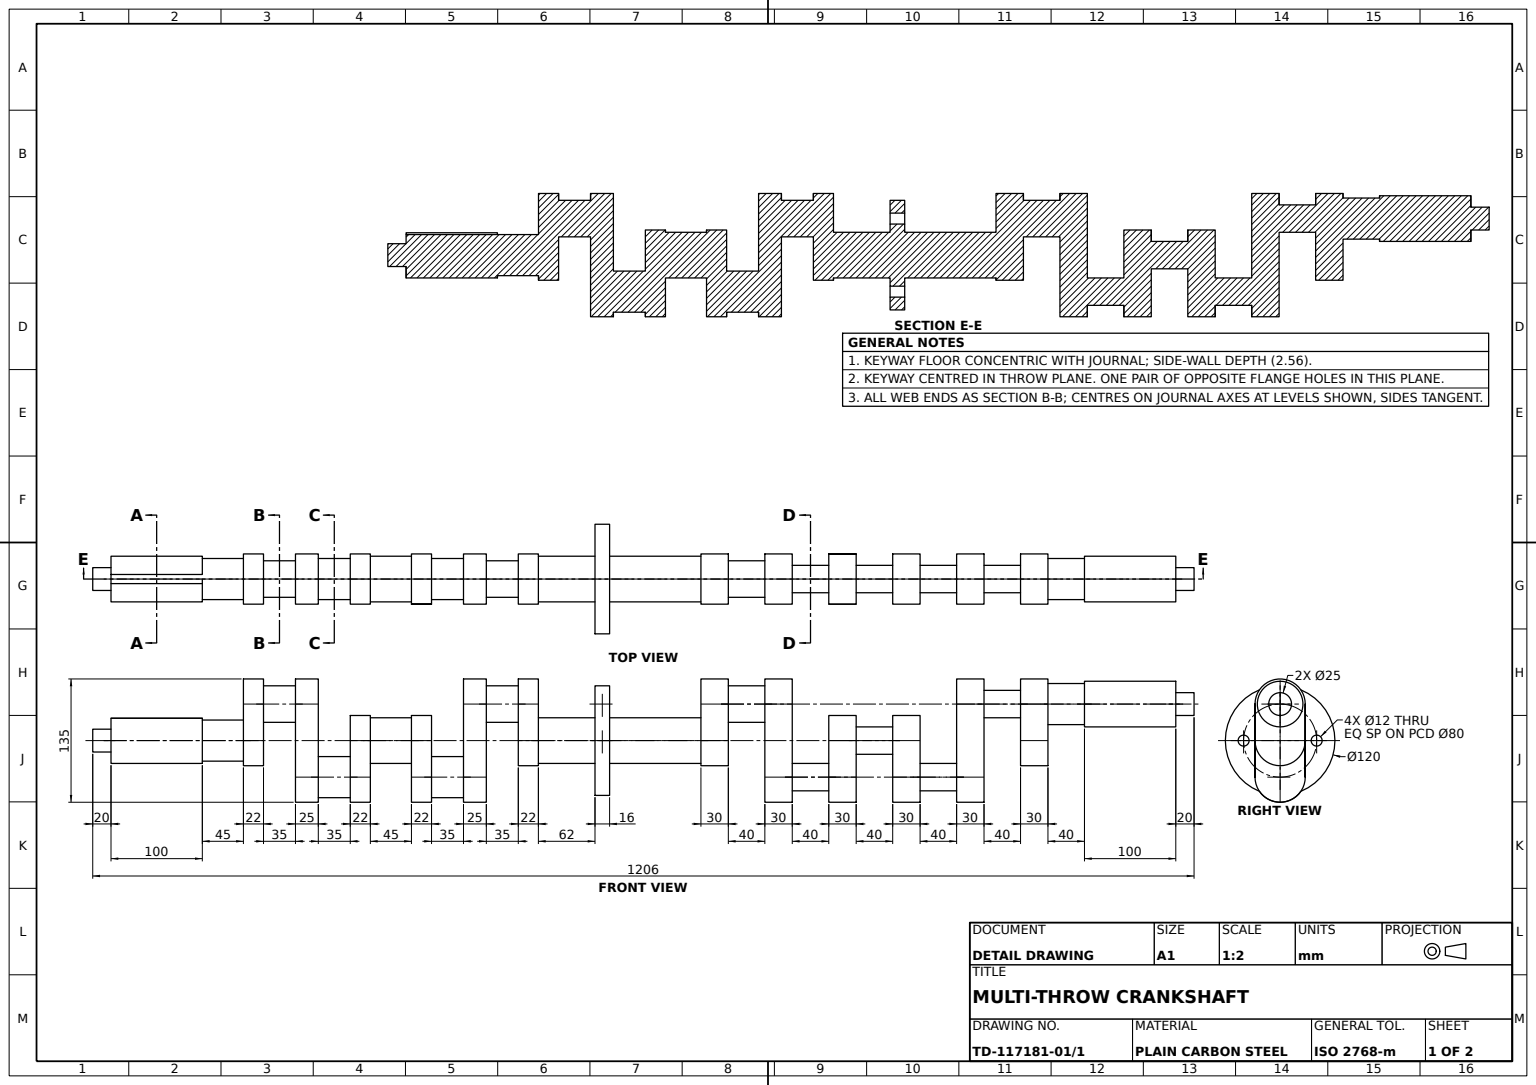
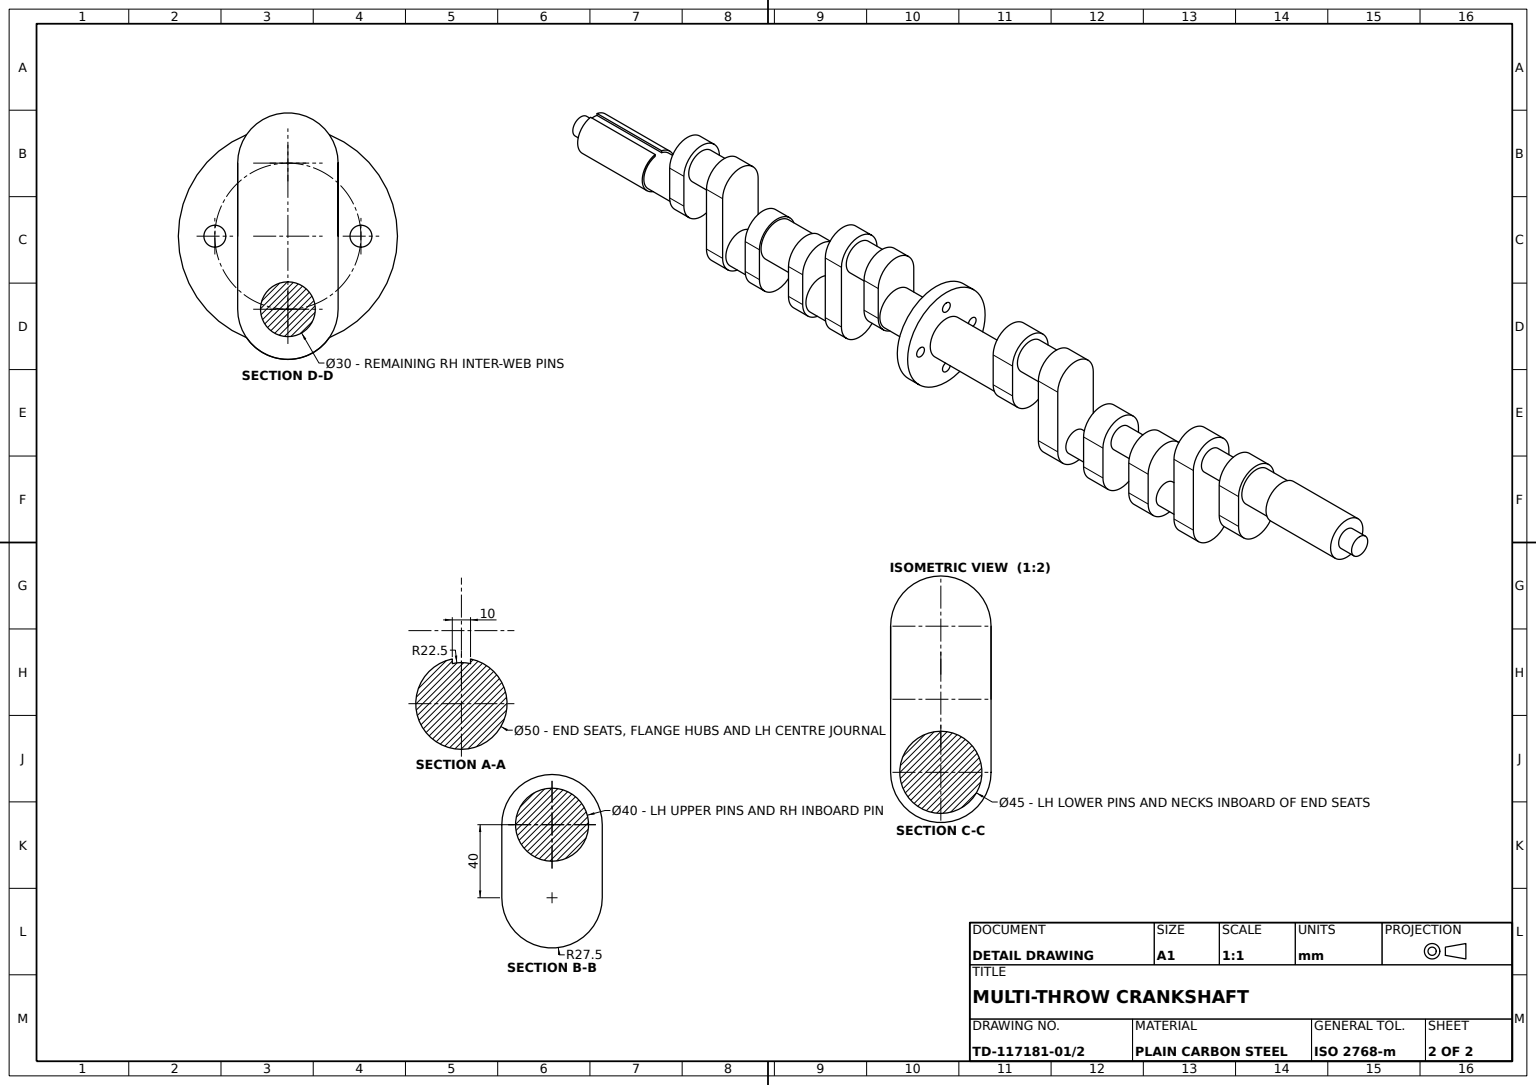
SolidWorks part; units mm, degrees
other "Markup1"
sketch "Sketch6"
material "Plain Carbon Steel"
ref_plane "Front Plane" through (0, 0, 0) normal (0, 0, 1) x (1, 0, 0)
ref_plane "Top Plane" through (0, 0, 0) normal (0, 1, 0) x (1, 0, 0)
ref_plane "Right Plane" through (0, 0, 0) normal (1, 0, 0) x (0, 0, -1)
sketch "Centre Flange Sketch" plane through (0, 0, 0) normal (0, 0, 1) x (1, 0, 0)
  circle A0 centre (0, 0) radius 60
  dimension "D1" = 120
extrude "Centre Flange Ø120" add sketch "Centre Flange Sketch" along normal blind 16
sketch "Flange Holes Sketch" plane through (0, 0, 16) normal (0, 0, 1) x (1, 0, 0)
  line L0 (0, 60) -> (0, -60) construction
  line L1 (-60, 0) -> (60, 0) construction
  circle A1 centre (0, 0) radius 60 construction
  circle A2 centre (0, 40) radius 6
  circle A3 centre (40, 0) radius 6
  circle A4 centre (0, -40) radius 6
  circle A5 centre (-40, 0) radius 6
  point P1 (0, 0)
  dimension "D1" = 40
  dimension "D2" = 12
  dimension "D3" = 40
  dimension "D4" = 40
  dimension "D5" = 40
extrude "Flange Holes Ø12" cut sketch "Flange Holes Sketch" against normal through all
sketch "A Journal 1 Sketch" plane through (0, 0, 16) normal (0, 0, 1) x (1, 0, 0)
  circle A0 centre (0, 0) radius 25
  dimension "D1" = 50
extrude "A Journal 1 Ø50" add sketch "A Journal 1 Sketch" along normal blind 62
sketch "A Web 1 Sketch" plane through (0, 0, 78) normal (0, 0, 1) x (1, 0, 0)
  line L0 (0, 0) -> (-40, 0) construction
  line L1 (0, -27.5) -> (-40, -27.5)
  line L2 (0, 27.5) -> (-40, 27.5)
  arc A0 (0, -27.5) -> (0, 27.5) centre (0, 0) ccw
  arc A1 (-40, 27.5) -> (-40, -27.5) centre (-40, 0) ccw
  point P3 (-20, 0)
  dimension "D2" = 27.5
  dimension "D1" = 40
extrude "A Web 1" add sketch "A Web 1 Sketch" along normal blind 22
sketch "A Pin 1 Sketch" plane through (0, 0, 100) normal (0, 0, 1) x (1, 0, 0)
  line L0 (-40, -27.5) -> (-40, 27.5) construction
  circle A0 centre (-40, 0) radius 20
  dimension "D1" = 40
extrude "A Pin 1 Ø40" add sketch "A Pin 1 Sketch" along normal blind 35
sketch "A Web 2 Sketch" plane through (0, 0, 135) normal (0, 0, 1) x (1, 0, 0)
  line L0 (-40, 0) -> (40, 0) construction
  line L1 (-40, 27.5) -> (40, 27.5)
  line L2 (-40, -27.5) -> (40, -27.5)
  arc A0 (-40, 27.5) -> (-40, -27.5) centre (-40, 0) ccw
  arc A1 (40, -27.5) -> (40, 27.5) centre (40, 0) ccw
  point P4 (0, 0)
  dimension "D2" = 27.5
  dimension "D1" = 80
extrude "A Web 2" add sketch "A Web 2 Sketch" along normal blind 25
sketch "A Pin 2 Sketch" plane through (0, 0, 160) normal (0, 0, 1) x (1, 0, 0)
  line L0 (40, 27.5) -> (40, -27.5) construction
  arc A0 (40, -27.5) -> (40, 27.5) centre (40, 0) ccw construction
  circle A1 centre (40, 0) radius 22.5
  dimension "D1" = 45
  dimension "D2" = 40
extrude "A Pin 2 Ø45" add sketch "A Pin 2 Sketch" along normal blind 35
sketch "A Web 3 Sketch" plane through (0, 0, 195) normal (0, 0, 1) x (1, 0, 0)
  line L0 (40, 0) -> (0, 0) construction
  line L1 (40, -27.5) -> (0, -27.5)
  line L2 (40, 27.5) -> (0, 27.5)
  arc A0 (40, -27.5) -> (40, 27.5) centre (40, 0) ccw
  arc A1 (0, 27.5) -> (0, -27.5) centre (0, 0) ccw
  point P4 (20, 0)
  dimension "D2" = 27.5
  dimension "D1" = 40
extrude "A Web 3" add sketch "A Web 3 Sketch" along normal blind 22
sketch "A Journal 2 Sketch" plane through (0, 0, 217) normal (0, 0, 1) x (1, 0, 0)
  circle A0 centre (0, 0) radius 25
  dimension "D1" = 50
extrude "A Journal 2 Ø50" add sketch "A Journal 2 Sketch" along normal blind 45
sketch "A Web 4 Sketch" plane through (0, 0, 262) normal (0, 0, 1) x (1, 0, 0)
  line L0 (0, 0) -> (40, 0) construction
  line L1 (0, 27.5) -> (40, 27.5)
  line L2 (0, -27.5) -> (40, -27.5)
  arc A0 (0, 27.5) -> (0, -27.5) centre (0, 0) ccw
  arc A1 (40, -27.5) -> (40, 27.5) centre (40, 0) ccw
  point P3 (20, 0)
  dimension "D2" = 27.5
  dimension "D1" = 40
extrude "A Web 4" add sketch "A Web 4 Sketch" along normal blind 22
sketch "A Pin 3 Sketch" plane through (0, 0, 284) normal (0, 0, 1) x (1, 0, 0)
  line L0 (40, 27.5) -> (40, -27.5) construction
  line L1 (0, -27.5) -> (40, -27.5) construction
  arc A0 (40, -27.5) -> (40, 27.5) centre (40, 0) ccw construction
  circle A1 centre (40, 0) radius 22.5
  dimension "D1" = 45
extrude "A Pin 3 Ø45" add sketch "A Pin 3 Sketch" along normal blind 35
sketch "A Web 5 Sketch" plane through (0, 0, 319) normal (0, 0, 1) x (1, 0, 0)
  line L0 (40, 0) -> (-40, 0) construction
  line L1 (40, -27.5) -> (-40, -27.5)
  line L2 (40, 27.5) -> (-40, 27.5)
  arc A0 (40, -27.5) -> (40, 27.5) centre (40, 0) ccw
  arc A1 (-40, 27.5) -> (-40, -27.5) centre (-40, 0) ccw
  point P3 (0, 0)
  dimension "D2" = 27.5
  dimension "D1" = 80
extrude "A Web 5" add sketch "A Web 5 Sketch" along normal blind 25
sketch "A Pin 4 Sketch" plane through (0, 0, 344) normal (0, 0, 1) x (1, 0, 0)
  line L0 (-40, 27.5) -> (-40, -27.5) construction
  arc A0 (-40, 27.5) -> (-40, -27.5) centre (-40, 0) ccw construction
  circle A1 centre (-40, 0) radius 20
  dimension "D1" = 40
extrude "A Pin 4 Ø40" add sketch "A Pin 4 Sketch" along normal blind 35
sketch "A Web 6 Sketch" plane through (0, 0, 379) normal (0, 0, 1) x (1, 0, 0)
  line L0 (-40, 0) -> (0, 0) construction
  line L1 (-40, 27.5) -> (0, 27.5)
  line L2 (-40, -27.5) -> (0, -27.5)
  arc A0 (-40, 27.5) -> (-40, -27.5) centre (-40, 0) ccw
  arc A1 (0, -27.5) -> (0, 27.5) centre (0, 0) ccw
  point P4 (-20, 0)
  dimension "D2" = 27.5
  dimension "D1" = 40
extrude "A Web 6" add sketch "A Web 6 Sketch" along normal blind 22
sketch "A Journal 3 Sketch" plane through (0, 0, 401) normal (0, 0, 1) x (1, 0, 0)
  circle A0 centre (0, 0) radius 22.5
  dimension "D1" = 45
extrude "A Journal 3 Ø45" add sketch "A Journal 3 Sketch" along normal blind 45
sketch "A Shaft End Sketch" plane through (0, 0, 446) normal (0, 0, 1) x (1, 0, 0)
  line L0 (0, 0) -> (-22.5, 0) construction
  line L2 (-24.4949, 5) -> (-21.9374, 5)
  line L4 (-21.9374, -5) -> (-24.4949, -5)
  arc A0 (-24.4949, -5) -> (-24.4949, 5) centre (0, 0) ccw
  arc A1 (-21.9374, 5) -> (-21.9374, -5) centre (0, 0) ccw
  dimension "D1" = 50
  dimension "D2" = 45
  dimension "D3" = 10
  dimension "D4" = 2.5575
extrude "A Shaft End" add sketch "A Shaft End Sketch" along normal blind 100
sketch "A End Spigot Sketch" plane through (0, 0, 546) normal (0, 0, 1) x (1, 0, 0)
  circle A0 centre (0, 0) radius 12.5
  dimension "D1" = 25
extrude "A End Spigot Ø25" add sketch "A End Spigot Sketch" along normal blind 20
sketch "B Journal 1 Sketch" plane through (0, 0, 0) normal (0, 0, -1) x (-1, 0, 0)
  circle A0 centre (0, 0) radius 25
  dimension "D1" = 50
extrude "B Journal 1 Ø50" add sketch "B Journal 1 Sketch" along normal blind 100
sketch "B Web 1 Sketch" plane through (0, 0, -100) normal (0, 0, -1) x (-1, 0, 0)
  line L0 (0, 0) -> (40, 0) construction
  line L1 (0, 27.5) -> (40, 27.5)
  line L2 (0, -27.5) -> (40, -27.5)
  arc A0 (0, 27.5) -> (0, -27.5) centre (0, 0) ccw
  arc A1 (40, -27.5) -> (40, 27.5) centre (40, 0) ccw
  point P3 (20, 0)
  dimension "D2" = 27.5
  dimension "D1" = 40
extrude "B Web 1" add sketch "B Web 1 Sketch" along normal blind 30
sketch "B Pin 1 Sketch" plane through (0, 0, -130) normal (0, 0, -1) x (-1, 0, 0)
  line L0 (40, 27.5) -> (40, -27.5) construction
  arc A0 (40, -27.5) -> (40, 27.5) centre (40, 0) ccw construction
  circle A1 centre (40, 0) radius 20
  dimension "D1" = 40
extrude "B Pin 1 Ø40" add sketch "B Pin 1 Sketch" along normal blind 40
sketch "B Web 2 Sketch" plane through (0, 0, -170) normal (0, 0, -1) x (-1, 0, 0)
  line L0 (40, 0) -> (-40, 0) construction
  line L1 (40, -27.5) -> (-40, -27.5)
  line L2 (40, 27.5) -> (-40, 27.5)
  arc A0 (40, -27.5) -> (40, 27.5) centre (40, 0) ccw
  arc A1 (-40, 27.5) -> (-40, -27.5) centre (-40, 0) ccw
  point P4 (0, 0)
  dimension "D2" = 27.5
  dimension "D1" = 80
extrude "B Web 2" add sketch "B Web 2 Sketch" along normal blind 30
sketch "B Journal 2 Sketch" plane through (0, 0, -200) normal (0, 0, -1) x (-1, 0, 0)
  circle A0 centre (-40, 0) radius 15
  dimension "D1" = 30
extrude "B Journal 2 Ø30" add sketch "B Journal 2 Sketch" along normal blind 40
sketch "B Web 3 Sketch" plane through (0, 0, -240) normal (0, 0, -1) x (-1, 0, 0)
  line L0 (-40, 0) -> (0, 0) construction
  line L1 (-40, 27.5) -> (0, 27.5)
  line L2 (-40, -27.5) -> (0, -27.5)
  arc A0 (-40, 27.5) -> (-40, -27.5) centre (-40, 0) ccw
  arc A1 (0, -27.5) -> (0, 27.5) centre (0, 0) ccw
  point P4 (-20, 0)
  dimension "D2" = 27.5
  dimension "D1" = 40
extrude "B Web 3" add sketch "B Web 3 Sketch" along normal blind 30
sketch "B Journal 3 Sketch" plane through (0, 0, -270) normal (0, 0, -1) x (-1, 0, 0)
  circle A0 centre (0, 0) radius 15
  dimension "D1" = 30
extrude "B Journal 3 Ø30" add sketch "B Journal 3 Sketch" along normal blind 40
sketch "B Web 4 Sketch" plane through (0, 0, -310) normal (0, 0, -1) x (-1, 0, 0)
  line L0 (0, 0) -> (-40, 0) construction
  line L1 (0, -27.5) -> (-40, -27.5)
  line L2 (0, 27.5) -> (-40, 27.5)
  arc A0 (0, -27.5) -> (0, 27.5) centre (0, 0) ccw
  arc A1 (-40, 27.5) -> (-40, -27.5) centre (-40, 0) ccw
  point P3 (-20, 0)
  dimension "D2" = 27.5
  dimension "D1" = 40
extrude "B Web 4" add sketch "B Web 4 Sketch" along normal blind 30
sketch "B Journal 4 Sketch" plane through (0, 0, -340) normal (0, 0, -1) x (-1, 0, 0)
  circle A0 centre (-40, 0) radius 15
  dimension "D1" = 30
extrude "B Journal 4 Ø30" add sketch "B Journal 4 Sketch" along normal blind 40
sketch "B Web 5 Sketch" plane through (0, 0, -380) normal (0, 0, -1) x (-1, 0, 0)
  line L0 (-40, 0) -> (40, 0) construction
  line L1 (-40, 27.5) -> (40, 27.5)
  line L2 (-40, -27.5) -> (40, -27.5)
  arc A0 (-40, 27.5) -> (-40, -27.5) centre (-40, 0) ccw
  arc A1 (40, -27.5) -> (40, 27.5) centre (40, 0) ccw
  point P4 (0, 0)
  dimension "D2" = 27.5
  dimension "D1" = 80
extrude "B Web 5" add sketch "B Web 5 Sketch" along normal blind 30
sketch "B Journal 5 Sketch" plane through (0, 0, -410) normal (0, 0, -1) x (-1, 0, 0)
  circle A0 centre (40, 0) radius 15
  dimension "D1" = 30
extrude "B Journal 5 Ø30" add sketch "B Journal 5 Sketch" along normal blind 40
sketch "B Web 6 Sketch" plane through (0, 0, -450) normal (0, 0, -1) x (-1, 0, 0)
  line L0 (40, 0) -> (0, 0) construction
  line L1 (40, -27.5) -> (0, -27.5)
  line L2 (40, 27.5) -> (0, 27.5)
  arc A0 (40, -27.5) -> (40, 27.5) centre (40, 0) ccw
  arc A1 (0, 27.5) -> (0, -27.5) centre (0, 0) ccw
  point P4 (20, 0)
  dimension "D2" = 27.5
  dimension "D1" = 40
extrude "B Web 6" add sketch "B Web 6 Sketch" along normal blind 30
sketch "B Journal 6 Sketch" plane through (0, 0, -480) normal (0, 0, -1) x (-1, 0, 0)
  circle A0 centre (40, 0) radius 22.5
  dimension "D1" = 45
extrude "B Journal 6 Ø45" add sketch "B Journal 6 Sketch" along normal blind 40
sketch "B Shaft End Sketch" plane through (0, 0, -520) normal (0, 0, -1) x (-1, 0, 0)
  circle A0 centre (40, 0) radius 25
  dimension "D1" = 50
extrude "B Shaft End Ø50" add sketch "B Shaft End Sketch" along normal blind 100
sketch "B End Spigot Sketch" plane through (0, 0, -620) normal (0, 0, -1) x (-1, 0, 0)
  circle A0 centre (40, 0) radius 12.5
  dimension "D1" = 25
extrude "B End Spigot Ø25" add sketch "B End Spigot Sketch" along normal blind 20
